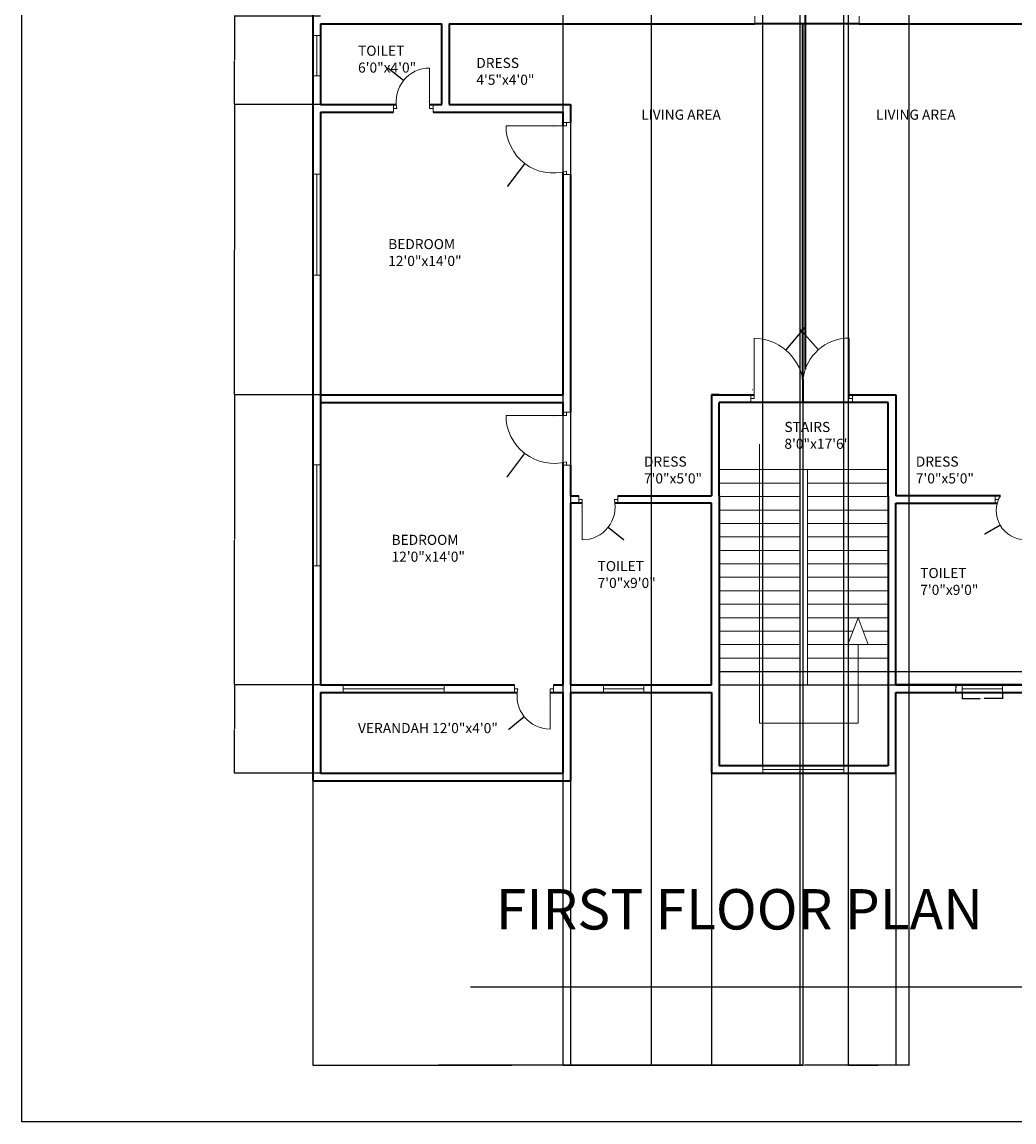
# Model space of a CAD drawing. Units: inches. Extents: x 1865 to 2795, y 1308 to 2437.
# Tile 1 of 3: x 1865 to 2455, y 1308 to 1962. Entities that reach past the tile are written whole.
import ezdxf

# ---------------------------------------------------------------- set-up
doc = ezdxf.new("R2010")
doc.units = ezdxf.units.IN
for name, color, linetype, lineweight in [('A-ANNO-DIMS', 2, 'Continuous', 18), ('A-ANNO-SYMB', 2, 'Continuous', 18), ('A-ANNO-TTLB', 7, 'Continuous', 25), ('A-AREA-IDEN', 7, 'Continuous', 18), ('A-DOOR', 3, 'Continuous', 18), ('A-FLOR-STRS', 7, 'Continuous', 18), ('A-GLAZ', 4, 'Continuous', 18), ('A-WALL', 7, 'Continuous', 35)]:
    doc.layers.add(name, color=color, linetype=linetype, lineweight=lineweight)
doc.styles.get("Standard").update_dxf_attribs({"font": 'arial.ttf'})
doc.dimstyles.get("Standard").update_dxf_attribs({"dimtxt": 0.18, "dimasz": 0.18, "dimexe": 0.18, "dimexo": 0.0625, "dimgap": 0.09, "dimtad": 0, "dimtih": 1, "dimtoh": 1, "dimdec": 4, "dimzin": 0, "dimdsep": 46, "dimtxsty": 'Standard', "dimcen": 0.09, "dimadec": 0, "dimazin": 0, "dimtfac": 1, "dimtdec": 4, "dimtofl": 0, "dimtmove": 0, "dimatfit": 3, "dimfxl": 1, "dimtolj": 1, "dimtzin": 0, "dimarcsym": 0})

# ---------------------------------------------------------------- blocks, each defined once
blk = doc.blocks.new('WIN-60IN')
for p, q in [((0, 4.5), (0, 0)), ((0, 0), (0, 2.25)), ((0, 2.25), (60, 2.25)), ((60, 2.25), (60, 4.5)), ((60, 4.5), (60, 0))]:
    blk.add_line(p, q)
blk = doc.blocks.new('WIN-60IN-ALT')
for p, q in [((4.5, 60), (0, 60)), ((0, 60), (2.25, 60)), ((2.25, 60), (2.25, 0)), ((2.25, 0), (0, 0)), ((0, 0), (4.5, 0))]:
    blk.add_line(p, q)
blk = doc.blocks.new('WIN-24IN')
for p, q in [((0, 24), (4.5, 24)), ((4.5, 24), (2.25, 24)), ((2.25, 24), (2.25, 0)), ((2.25, 0), (0, 0)), ((0, 0), (4.5, 0))]:
    blk.add_line(p, q)
blk = doc.blocks.new('*D6')
at = {"layer": 'A-ANNO-DIMS', "color": 0, "lineweight": -2, "transparency": 16777216}
for p, q in [((2424.19, 1563.59), (2424.19, 1559.88)), ((2448.19, 1563.59), (2448.19, 1559.88)), ((2424.37, 1560.06), (2435.07, 1560.06)), ((2448.01, 1560.06), (2437.31, 1560.06))]:
    blk.add_line(p, q, dxfattribs=at)
at = {"layer": 'A-ANNO-DIMS', "color": 0, "transparency": 16777216}
for points in [[(2424.37, 1560.09), (2424.37, 1560.03), (2424.19, 1560.06)], [(2448.01, 1560.09), (2448.01, 1560.03), (2448.19, 1560.06)]]:
    blk.add_solid(points, dxfattribs=at)
at = {"layer": 'Defpoints', "color": 0, "transparency": 16777216}
for p in [(2424.19, 1563.66), (2448.19, 1563.66), (2448.19, 1560.06)]:
    blk.add_point(p, dxfattribs=at)
at = {"layer": 'A-ANNO-DIMS', "color": 0, "transparency": 16777216, "insert": (2436.19, 1560.06), "char_height": 0.18, "attachment_point": 5}
blk.add_mtext('\\A1;WINDOW 24 TYP.', dxfattribs=at)
blk = doc.blocks.new('*D7')
at = {"layer": 'A-ANNO-DIMS', "color": 0, "lineweight": -2, "transparency": 16777216}
for p, q in [((2424.13, 1568.16), (2420.41, 1568.16)), ((2424.13, 1563.66), (2420.41, 1563.66)), ((2420.59, 1567.98), (2420.59, 1566.09)), ((2420.59, 1563.84), (2420.59, 1565.72))]:
    blk.add_line(p, q, dxfattribs=at)
at = {"layer": 'A-ANNO-DIMS', "color": 0, "transparency": 16777216}
for points in [[(2420.56, 1567.98), (2420.62, 1567.98), (2420.59, 1568.16)], [(2420.56, 1563.84), (2420.62, 1563.84), (2420.59, 1563.66)]]:
    blk.add_solid(points, dxfattribs=at)
at = {"layer": 'Defpoints', "color": 0, "transparency": 16777216}
for p in [(2420.59, 1563.66), (2424.19, 1568.16), (2424.19, 1563.66)]:
    blk.add_point(p, dxfattribs=at)
at = {"layer": 'A-ANNO-DIMS', "color": 0, "transparency": 16777216, "insert": (2420.59, 1565.91), "char_height": 0.18, "attachment_point": 5}
blk.add_mtext('\\A1;5 TYP.', dxfattribs=at)
blk = doc.blocks.new('*D12')
at = {"layer": 'A-ANNO-DIMS', "color": 0, "lineweight": -2, "transparency": 16777216}
for p, q in [((2038.34, 2310.59), (2038.34, 1341.86)), ((2186.84, 2306.09), (2186.84, 1341.86)), ((2038.52, 1342.04), (2112.2, 1342.04)), ((2186.66, 1342.04), (2112.97, 1342.04))]:
    blk.add_line(p, q, dxfattribs=at)
at = {"layer": 'A-ANNO-DIMS', "color": 0, "transparency": 16777216}
for points in [[(2038.52, 1342.07), (2038.52, 1342.01), (2038.34, 1342.04)], [(2186.66, 1342.07), (2186.66, 1342.01), (2186.84, 1342.04)]]:
    blk.add_solid(points, dxfattribs=at)
at = {"layer": 'Defpoints', "color": 0, "transparency": 16777216}
for p in [(2038.34, 2310.66), (2186.84, 2306.16), (2186.84, 1342.04)]:
    blk.add_point(p, dxfattribs=at)
at = {"layer": 'A-ANNO-DIMS', "color": 0, "transparency": 16777216, "insert": (2112.59, 1342.04), "char_height": 0.18, "attachment_point": 5}
blk.add_mtext('\\A1;148.5', dxfattribs=at)
blk = doc.blocks.new('*D13')
at = {"layer": 'A-ANNO-DIMS', "color": 0, "lineweight": -2, "transparency": 16777216}
for p, q in [((2186.84, 2306.09), (2186.84, 1341.86)), ((2239.34, 2306.09), (2239.34, 1341.86)), ((2187.02, 1342.04), (2212.76, 1342.04)), ((2239.16, 1342.04), (2213.41, 1342.04))]:
    blk.add_line(p, q, dxfattribs=at)
at = {"layer": 'A-ANNO-DIMS', "color": 0, "transparency": 16777216}
for points in [[(2187.02, 1342.07), (2187.02, 1342.01), (2186.84, 1342.04)], [(2239.16, 1342.07), (2239.16, 1342.01), (2239.34, 1342.04)]]:
    blk.add_solid(points, dxfattribs=at)
at = {"layer": 'Defpoints', "color": 0, "transparency": 16777216}
for p in [(2186.84, 2306.16), (2239.34, 2306.16), (2239.34, 1342.04)]:
    blk.add_point(p, dxfattribs=at)
at = {"layer": 'A-ANNO-DIMS', "color": 0, "transparency": 16777216, "insert": (2213.09, 1342.04), "char_height": 0.18, "attachment_point": 5}
blk.add_mtext('\\A1;52.5', dxfattribs=at)
blk = doc.blocks.new('*D14')
at = {"layer": 'A-ANNO-DIMS', "color": 0, "lineweight": -2, "transparency": 16777216}
for p, q in [((2239.34, 2306.09), (2239.34, 1341.86)), ((2327.84, 2306.09), (2327.84, 1341.86)), ((2239.52, 1342.04), (2283.26, 1342.04)), ((2327.66, 1342.04), (2283.91, 1342.04))]:
    blk.add_line(p, q, dxfattribs=at)
at = {"layer": 'A-ANNO-DIMS', "color": 0, "transparency": 16777216}
for points in [[(2239.52, 1342.07), (2239.52, 1342.01), (2239.34, 1342.04)], [(2327.66, 1342.07), (2327.66, 1342.01), (2327.84, 1342.04)]]:
    blk.add_solid(points, dxfattribs=at)
at = {"layer": 'Defpoints', "color": 0, "transparency": 16777216}
for p in [(2239.34, 2306.16), (2327.84, 2306.16), (2327.84, 1342.04)]:
    blk.add_point(p, dxfattribs=at)
at = {"layer": 'A-ANNO-DIMS', "color": 0, "transparency": 16777216, "insert": (2283.59, 1342.04), "char_height": 0.18, "attachment_point": 5}
blk.add_mtext('\\A1;88.5', dxfattribs=at)
blk = doc.blocks.new('*D18')
at = {"layer": 'A-ANNO-DIMS', "color": 0, "lineweight": -2, "transparency": 16777216}
for p, q in [((2356.56, 2306.09), (2356.56, 1341.86)), ((2392.56, 2306.09), (2392.56, 1341.86)), ((2356.74, 1342.04), (2374.34, 1342.04)), ((2392.38, 1342.04), (2374.78, 1342.04))]:
    blk.add_line(p, q, dxfattribs=at)
at = {"layer": 'A-ANNO-DIMS', "color": 0, "transparency": 16777216}
for points in [[(2356.74, 1342.07), (2356.74, 1342.01), (2356.56, 1342.04)], [(2392.38, 1342.07), (2392.38, 1342.01), (2392.56, 1342.04)]]:
    blk.add_solid(points, dxfattribs=at)
at = {"layer": 'Defpoints', "color": 0, "transparency": 16777216}
for p in [(2356.56, 2306.16), (2392.56, 2306.16), (2392.56, 1342.04)]:
    blk.add_point(p, dxfattribs=at)
at = {"layer": 'A-ANNO-DIMS', "color": 0, "transparency": 16777216, "insert": (2374.56, 1342.04), "char_height": 0.18, "attachment_point": 5}
blk.add_mtext('\\A1;36', dxfattribs=at)
blk = doc.blocks.new('*D19')
at = {"layer": 'A-ANNO-DIMS', "color": 0, "lineweight": -2, "transparency": 16777216}
for p, q in [((2305.85, 1520.22), (2305.85, 2357.44)), ((2306.03, 2357.26), (2329.63, 2357.26)), ((2353.67, 2357.26), (2330.08, 2357.26)), ((2353.85, 1520.22), (2353.85, 2357.44))]:
    blk.add_line(p, q, dxfattribs=at)
at = {"layer": 'A-ANNO-DIMS', "color": 0, "transparency": 16777216}
for points in [[(2306.03, 2357.29), (2306.03, 2357.23), (2305.85, 2357.26)], [(2353.67, 2357.29), (2353.67, 2357.23), (2353.85, 2357.26)]]:
    blk.add_solid(points, dxfattribs=at)
at = {"layer": 'Defpoints', "color": 0, "transparency": 16777216}
for p in [(2353.85, 2357.26), (2305.85, 1520.16), (2353.85, 1520.16)]:
    blk.add_point(p, dxfattribs=at)
at = {"layer": 'A-ANNO-DIMS', "color": 0, "transparency": 16777216, "insert": (2329.85, 2357.26), "char_height": 0.18, "attachment_point": 5}
blk.add_mtext('\\A1;48', dxfattribs=at)
blk = doc.blocks.new('*D20')
at = {"layer": 'A-ANNO-DIMS', "color": 0, "lineweight": -2, "transparency": 16777216}
for p, q in [((2042.78, 1568.16), (1991.56, 1568.16)), ((1991.74, 1567.98), (1991.74, 1542.09)), ((1991.74, 1515.84), (1991.74, 1541.72)), ((2042.78, 1515.66), (1991.56, 1515.66))]:
    blk.add_line(p, q, dxfattribs=at)
at = {"layer": 'A-ANNO-DIMS', "color": 0, "transparency": 16777216}
for points in [[(1991.71, 1567.98), (1991.77, 1567.98), (1991.74, 1568.16)], [(1991.71, 1515.84), (1991.77, 1515.84), (1991.74, 1515.66)]]:
    blk.add_solid(points, dxfattribs=at)
at = {"layer": 'Defpoints', "color": 0, "transparency": 16777216}
for p in [(1991.74, 1568.16), (2042.84, 1568.16), (2042.84, 1515.66)]:
    blk.add_point(p, dxfattribs=at)
at = {"layer": 'A-ANNO-DIMS', "color": 0, "transparency": 16777216, "insert": (1991.74, 1541.91), "char_height": 0.18, "attachment_point": 5}
blk.add_mtext('\\A1;52.5', dxfattribs=at)
blk = doc.blocks.new('*D21')
at = {"layer": 'A-ANNO-DIMS', "color": 0, "lineweight": -2, "transparency": 16777216}
for p, q in [((2042.78, 1740.66), (1991.56, 1740.66)), ((1991.74, 1740.48), (1991.74, 1654.59)), ((1991.74, 1568.34), (1991.74, 1654.22)), ((2042.78, 1568.16), (1991.56, 1568.16))]:
    blk.add_line(p, q, dxfattribs=at)
at = {"layer": 'A-ANNO-DIMS', "color": 0, "transparency": 16777216}
for points in [[(1991.71, 1740.48), (1991.77, 1740.48), (1991.74, 1740.66)], [(1991.71, 1568.34), (1991.77, 1568.34), (1991.74, 1568.16)]]:
    blk.add_solid(points, dxfattribs=at)
at = {"layer": 'Defpoints', "color": 0, "transparency": 16777216}
for p in [(1991.74, 1740.66), (2042.84, 1740.66), (2042.84, 1568.16)]:
    blk.add_point(p, dxfattribs=at)
at = {"layer": 'A-ANNO-DIMS', "color": 0, "transparency": 16777216, "insert": (1991.74, 1654.41), "char_height": 0.18, "attachment_point": 5}
blk.add_mtext('\\A1;172.5', dxfattribs=at)
blk = doc.blocks.new('*D22')
at = {"layer": 'A-ANNO-DIMS', "color": 0, "lineweight": -2, "transparency": 16777216}
for p, q in [((2042.78, 1913.16), (1991.56, 1913.16)), ((1991.74, 1912.98), (1991.74, 1827.09)), ((1991.74, 1740.84), (1991.74, 1826.72)), ((2042.78, 1740.66), (1991.56, 1740.66))]:
    blk.add_line(p, q, dxfattribs=at)
at = {"layer": 'A-ANNO-DIMS', "color": 0, "transparency": 16777216}
for points in [[(1991.71, 1912.98), (1991.77, 1912.98), (1991.74, 1913.16)], [(1991.71, 1740.84), (1991.77, 1740.84), (1991.74, 1740.66)]]:
    blk.add_solid(points, dxfattribs=at)
at = {"layer": 'Defpoints', "color": 0, "transparency": 16777216}
for p in [(1991.74, 1913.16), (2042.84, 1913.16), (2042.84, 1740.66)]:
    blk.add_point(p, dxfattribs=at)
at = {"layer": 'A-ANNO-DIMS', "color": 0, "transparency": 16777216, "insert": (1991.74, 1826.91), "char_height": 0.18, "attachment_point": 5}
blk.add_mtext('\\A1;172.5', dxfattribs=at)
blk = doc.blocks.new('*D23')
at = {"layer": 'A-ANNO-DIMS', "color": 0, "lineweight": -2, "transparency": 16777216}
for p, q in [((2042.78, 1965.66), (1991.56, 1965.66)), ((1991.74, 1965.48), (1991.74, 1939.59)), ((1991.74, 1913.34), (1991.74, 1939.22)), ((2042.78, 1913.16), (1991.56, 1913.16))]:
    blk.add_line(p, q, dxfattribs=at)
at = {"layer": 'A-ANNO-DIMS', "color": 0, "transparency": 16777216}
for points in [[(1991.71, 1965.48), (1991.77, 1965.48), (1991.74, 1965.66)], [(1991.71, 1913.34), (1991.77, 1913.34), (1991.74, 1913.16)]]:
    blk.add_solid(points, dxfattribs=at)
at = {"layer": 'Defpoints', "color": 0, "transparency": 16777216}
for p in [(1991.74, 1965.66), (2042.84, 1965.66), (2042.84, 1913.16)]:
    blk.add_point(p, dxfattribs=at)
at = {"layer": 'A-ANNO-DIMS', "color": 0, "transparency": 16777216, "insert": (1991.74, 1939.41), "char_height": 0.18, "attachment_point": 5}
blk.add_mtext('\\A1;52.5', dxfattribs=at)
blk = doc.blocks.new('*D25')
at = {"layer": 'A-ANNO-DIMS', "color": 0, "lineweight": -2, "transparency": 16777216}
for p, q in [((2038.34, 1511.09), (2038.34, 1341.86)), ((2275.34, 1515.59), (2275.34, 1341.86)), ((2038.52, 1342.04), (2156.55, 1342.04)), ((2275.16, 1342.04), (2157.13, 1342.04))]:
    blk.add_line(p, q, dxfattribs=at)
at = {"layer": 'A-ANNO-DIMS', "color": 0, "transparency": 16777216}
for points in [[(2038.52, 1342.07), (2038.52, 1342.01), (2038.34, 1342.04)], [(2275.16, 1342.07), (2275.16, 1342.01), (2275.34, 1342.04)]]:
    blk.add_solid(points, dxfattribs=at)
at = {"layer": 'Defpoints', "color": 0, "transparency": 16777216}
for p in [(2038.34, 1511.16), (2275.34, 1515.66), (2275.34, 1342.04)]:
    blk.add_point(p, dxfattribs=at)
at = {"layer": 'A-ANNO-DIMS', "color": 0, "transparency": 16777216, "insert": (2156.84, 1342.04), "char_height": 0.18, "attachment_point": 5}
blk.add_mtext('\\A1;237', dxfattribs=at)
blk = doc.blocks.new('*D26')
at = {"layer": 'A-ANNO-DIMS', "color": 0, "lineweight": -2, "transparency": 16777216}
for p, q in [((2275.34, 1515.59), (2275.34, 1341.86)), ((2384.84, 1515.59), (2384.84, 1341.86)), ((2275.52, 1342.04), (2329.7, 1342.04)), ((2384.66, 1342.04), (2330.47, 1342.04))]:
    blk.add_line(p, q, dxfattribs=at)
at = {"layer": 'A-ANNO-DIMS', "color": 0, "transparency": 16777216}
for points in [[(2275.52, 1342.07), (2275.52, 1342.01), (2275.34, 1342.04)], [(2384.66, 1342.07), (2384.66, 1342.01), (2384.84, 1342.04)]]:
    blk.add_solid(points, dxfattribs=at)
at = {"layer": 'Defpoints', "color": 0, "transparency": 16777216}
for p in [(2275.34, 1515.66), (2384.84, 1515.66), (2384.84, 1342.04)]:
    blk.add_point(p, dxfattribs=at)
at = {"layer": 'A-ANNO-DIMS', "color": 0, "transparency": 16777216, "insert": (2330.09, 1342.04), "char_height": 0.18, "attachment_point": 5}
blk.add_mtext('\\A1;109.5', dxfattribs=at)
blk = doc.blocks.new('*D27')
at = {"layer": 'A-ANNO-DIMS', "color": 0, "lineweight": -2, "transparency": 16777216}
for p, q in [((2329.63, 1961.09), (2329.63, 1341.86)), ((2191.34, 1913.09), (2191.34, 1341.86)), ((2191.52, 1342.04), (2260.1, 1342.04)), ((2329.45, 1342.04), (2260.87, 1342.04))]:
    blk.add_line(p, q, dxfattribs=at)
at = {"layer": 'A-ANNO-DIMS', "color": 0, "transparency": 16777216}
for points in [[(2191.52, 1342.07), (2191.52, 1342.01), (2191.34, 1342.04)], [(2329.45, 1342.07), (2329.45, 1342.01), (2329.63, 1342.04)]]:
    blk.add_solid(points, dxfattribs=at)
at = {"layer": 'Defpoints', "color": 0, "transparency": 16777216}
for p in [(2329.63, 1961.16), (2191.34, 1913.16), (2329.63, 1342.04)]:
    blk.add_point(p, dxfattribs=at)
at = {"layer": 'A-ANNO-DIMS', "color": 0, "transparency": 16777216, "insert": (2260.48, 1342.04), "char_height": 0.18, "attachment_point": 5}
blk.add_mtext('\\A1;138.3', dxfattribs=at)
blk = doc.blocks.new('*D28')
at = {"layer": 'A-ANNO-DIMS', "color": 0, "lineweight": -2, "transparency": 16777216}
for p, q in [((2279.9, 1576.16), (2668.62, 1576.16)), ((2668.44, 1575.98), (2668.44, 1572.34)), ((2668.44, 1568.34), (2668.44, 1571.97)), ((2279.9, 1568.16), (2668.62, 1568.16))]:
    blk.add_line(p, q, dxfattribs=at)
at = {"layer": 'A-ANNO-DIMS', "color": 0, "transparency": 16777216}
for points in [[(2668.41, 1575.98), (2668.47, 1575.98), (2668.44, 1576.16)], [(2668.41, 1568.34), (2668.47, 1568.34), (2668.44, 1568.16)]]:
    blk.add_solid(points, dxfattribs=at)
at = {"layer": 'Defpoints', "color": 0, "transparency": 16777216}
for p in [(2279.84, 1576.16), (2668.44, 1576.16), (2279.84, 1568.16)]:
    blk.add_point(p, dxfattribs=at)
at = {"layer": 'A-ANNO-DIMS', "color": 0, "transparency": 16777216, "insert": (2668.44, 1572.16), "char_height": 0.18, "attachment_point": 5}
blk.add_mtext('\\A1;8', dxfattribs=at)
blk = doc.blocks.new('*D30')
at = {"layer": 'A-ANNO-DIMS', "color": 0, "lineweight": -2, "transparency": 16777216}
for p, q in [((2331.21, 1781.26), (2319.48, 1767.35)), ((2331.39, 1781.26), (2331.21, 1781.26)), ((2299.55, 1743.81), (2299.73, 1743.81)), ((2299.64, 1743.72), (2299.64, 1743.9))]:
    blk.add_line(p, q, dxfattribs=at)
at = {"layer": 'A-ANNO-DIMS', "color": 0, "transparency": 16777216}
blk.add_solid([(2319.46, 1767.37), (2319.51, 1767.34), (2319.37, 1767.22)], dxfattribs=at)
at = {"layer": 'Defpoints', "color": 0, "transparency": 16777216}
for p in [(2319.37, 1767.22), (2299.64, 1743.81)]:
    blk.add_point(p, dxfattribs=at)
at = {"layer": 'A-ANNO-DIMS', "color": 0, "transparency": 16777216, "insert": (2331.85, 1781.26), "char_height": 0.18, "attachment_point": 5}
blk.add_mtext('\\A1;R30.61', dxfattribs=at)
blk = doc.blocks.new('*D34')
at = {"layer": 'A-ANNO-DIMS', "color": 0, "lineweight": -2, "transparency": 16777216}
for p, q in [((2181.53, 1728.42), (2181.71, 1728.42)), ((2181.62, 1728.33), (2181.62, 1728.51)), ((2153.89, 1692.16), (2164.18, 1705.61)), ((2153.71, 1692.16), (2153.89, 1692.16))]:
    blk.add_line(p, q, dxfattribs=at)
at = {"layer": 'A-ANNO-DIMS', "color": 0, "transparency": 16777216}
blk.add_solid([(2164.15, 1705.63), (2164.2, 1705.59), (2164.29, 1705.76)], dxfattribs=at)
at = {"layer": 'Defpoints', "color": 0, "transparency": 16777216}
for p in [(2181.62, 1728.42), (2164.29, 1705.76)]:
    blk.add_point(p, dxfattribs=at)
at = {"layer": 'A-ANNO-DIMS', "color": 0, "transparency": 16777216, "insert": (2153.23, 1692.16), "char_height": 0.18, "attachment_point": 5}
blk.add_mtext('\\A1;R28.53', dxfattribs=at)
blk = doc.blocks.new('*D36')
at = {"layer": 'A-ANNO-DIMS', "color": 0, "lineweight": -2, "transparency": 16777216}
for p, q in [((2181.07, 1900.57), (2181.25, 1900.57)), ((2181.16, 1900.48), (2181.16, 1900.66)), ((2154.25, 1864.6), (2164.24, 1877.95)), ((2154.07, 1864.6), (2154.25, 1864.6))]:
    blk.add_line(p, q, dxfattribs=at)
at = {"layer": 'A-ANNO-DIMS', "color": 0, "transparency": 16777216}
blk.add_solid([(2164.21, 1877.96), (2164.26, 1877.93), (2164.34, 1878.09)], dxfattribs=at)
at = {"layer": 'Defpoints', "color": 0, "transparency": 16777216}
for p in [(2181.16, 1900.57), (2164.34, 1878.09)]:
    blk.add_point(p, dxfattribs=at)
at = {"layer": 'A-ANNO-DIMS', "color": 0, "transparency": 16777216, "insert": (2153.52, 1864.6), "char_height": 0.18, "attachment_point": 5}
blk.add_mtext('\\A1;R28.075', dxfattribs=at)
blk = doc.blocks.new('*D38')
at = {"layer": 'A-ANNO-DIMS', "color": 0, "lineweight": -2, "transparency": 16777216}
for p, q in [((2327.53, 1779.86), (2327.71, 1779.86)), ((2327.71, 1779.86), (2338.64, 1767.55)), ((2357.08, 1746.67), (2357.26, 1746.67)), ((2357.17, 1746.58), (2357.17, 1746.76))]:
    blk.add_line(p, q, dxfattribs=at)
at = {"layer": 'A-ANNO-DIMS', "color": 0, "transparency": 16777216}
blk.add_solid([(2338.66, 1767.57), (2338.61, 1767.53), (2338.76, 1767.42)], dxfattribs=at)
at = {"layer": 'Defpoints', "color": 0, "transparency": 16777216}
for p in [(2338.76, 1767.42), (2357.17, 1746.67)]:
    blk.add_point(p, dxfattribs=at)
at = {"layer": 'A-ANNO-DIMS', "color": 0, "transparency": 16777216, "insert": (2327.05, 1779.86), "char_height": 0.18, "attachment_point": 5}
blk.add_mtext('\\A1;R27.74', dxfattribs=at)
blk = doc.blocks.new('*D44')
at = {"layer": 'A-ANNO-DIMS', "color": 0, "lineweight": -2, "transparency": 16777216}
for p, q in [((2082.75, 1935.12), (2082.93, 1935.12)), ((2082.93, 1935.12), (2092.08, 1927.67)), ((2107.6, 1914.94), (2107.78, 1914.94)), ((2107.69, 1914.85), (2107.69, 1915.03))]:
    blk.add_line(p, q, dxfattribs=at)
at = {"layer": 'A-ANNO-DIMS', "color": 0, "transparency": 16777216}
blk.add_solid([(2092.09, 1927.69), (2092.06, 1927.64), (2092.22, 1927.55)], dxfattribs=at)
at = {"layer": 'Defpoints', "color": 0, "transparency": 16777216}
for p in [(2092.22, 1927.55), (2107.69, 1914.94)]:
    blk.add_point(p, dxfattribs=at)
at = {"layer": 'A-ANNO-DIMS', "color": 0, "transparency": 16777216, "insert": (2082.2, 1935.12), "char_height": 0.18, "attachment_point": 5}
blk.add_mtext('\\A1;R19.965', dxfattribs=at)
blk = doc.blocks.new('*D45')
at = {"layer": 'A-ANNO-DIMS', "color": 0, "lineweight": -2, "transparency": 16777216}
for p, q in [((2198.34, 1673.97), (2198.34, 1674.15)), ((2198.25, 1674.06), (2198.43, 1674.06)), ((2222.91, 1654.44), (2213.84, 1661.68)), ((2223.09, 1654.44), (2222.91, 1654.44))]:
    blk.add_line(p, q, dxfattribs=at)
at = {"layer": 'A-ANNO-DIMS', "color": 0, "transparency": 16777216}
blk.add_solid([(2213.86, 1661.71), (2213.82, 1661.66), (2213.7, 1661.8)], dxfattribs=at)
at = {"layer": 'Defpoints', "color": 0, "transparency": 16777216}
for p in [(2198.34, 1674.06), (2213.7, 1661.8)]:
    blk.add_point(p, dxfattribs=at)
at = {"layer": 'A-ANNO-DIMS', "color": 0, "transparency": 16777216, "insert": (2223.57, 1654.44), "char_height": 0.18, "attachment_point": 5}
blk.add_mtext('\\A1;R19.65', dxfattribs=at)
blk = doc.blocks.new('*D46')
at = {"layer": 'A-ANNO-DIMS', "color": 0, "lineweight": -2, "transparency": 16777216}
for p, q in [((2179.17, 1561.52), (2179.35, 1561.52)), ((2179.26, 1561.43), (2179.26, 1561.61)), ((2154.72, 1541.97), (2163.78, 1549.19)), ((2154.54, 1541.97), (2154.72, 1541.97))]:
    blk.add_line(p, q, dxfattribs=at)
at = {"layer": 'A-ANNO-DIMS', "color": 0, "transparency": 16777216}
blk.add_solid([(2163.76, 1549.21), (2163.8, 1549.16), (2163.92, 1549.3)], dxfattribs=at)
at = {"layer": 'Defpoints', "color": 0, "transparency": 16777216}
for p in [(2179.26, 1561.52), (2163.92, 1549.3)]:
    blk.add_point(p, dxfattribs=at)
at = {"layer": 'A-ANNO-DIMS', "color": 0, "transparency": 16777216, "insert": (2153.99, 1541.97), "char_height": 0.18, "attachment_point": 5}
blk.add_mtext('\\A1;R19.615', dxfattribs=at)
blk = doc.blocks.new('*D49')
at = {"layer": 'A-ANNO-DIMS', "color": 0, "lineweight": -2, "transparency": 16777216}
for p, q in [((2461.87, 1671.78), (2462.05, 1671.78)), ((2461.96, 1671.69), (2461.96, 1671.87)), ((2437.81, 1658.01), (2446.71, 1663.08)), ((2437.63, 1658.01), (2437.81, 1658.01))]:
    blk.add_line(p, q, dxfattribs=at)
at = {"layer": 'A-ANNO-DIMS', "color": 0, "transparency": 16777216}
blk.add_solid([(2446.7, 1663.11), (2446.73, 1663.06), (2446.87, 1663.17)], dxfattribs=at)
at = {"layer": 'Defpoints', "color": 0, "transparency": 16777216}
for p in [(2461.96, 1671.78), (2446.87, 1663.17)]:
    blk.add_point(p, dxfattribs=at)
at = {"layer": 'A-ANNO-DIMS', "color": 0, "transparency": 16777216, "insert": (2437.09, 1658.01), "char_height": 0.18, "attachment_point": 5}
blk.add_mtext('\\A1;R17.372', dxfattribs=at)

msp = doc.modelspace()

# ---------------------------------------------------------------- linework, layer by layer
at = {"layer": 'A-ANNO-SYMB'}
for p, q in [((2303.8379, 1711.3839), (2303.8379, 1545.3723)), ((2362.5426, 1608.1564), (2356.3379, 1592.1564)), ((2368.4808, 1592.1564), (2362.5426, 1608.1564)), ((2356.3379, 1592.1564), (2368.4808, 1592.1564)), ((2362.5426, 1545.3723), (2362.5426, 1592.1564)), ((2303.8379, 1545.3723), (2362.5426, 1545.3723))]:
    msp.add_line(p, q, dxfattribs=at)
at = {"layer": 'A-ANNO-TTLB'}
msp.add_line((2132.0289, 1388.6384), (2475.3371, 1388.6384), dxfattribs=at)
msp.add_lwpolyline([(1865.3404, 2436.9121), (2795.2369, 2436.9121), (2795.2369, 1308.3367), (1865.3404, 1308.3367)], close=True, dxfattribs=at)
at = {"layer": 'A-DOOR'}
for p, q in [((2301.0168, 1965.6564), (2301.0168, 1961.1564)), ((2301.0168, 1961.1564), (2301.0168, 1963.4064)), ((2363.0176, 1965.6564), (2363.0176, 1961.1564)), ((2363.0176, 1961.1564), (2363.0176, 1963.4064)), ((2107.6934, 1910.9064), (2107.6934, 1934.9064)), ((2086.1404, 1913.1564), (2086.1404, 1908.6564)), ((2086.1404, 1908.6564), (2086.1404, 1910.9064)), ((2086.1404, 1910.9064), (2088.1404, 1910.9064)), ((2109.6934, 1910.9064), (2107.6934, 1910.9064)), ((2109.6934, 1913.1564), (2109.6934, 1908.6564)), ((2109.6934, 1908.6564), (2109.6934, 1910.9064)), ((2189.0879, 1900.57), (2153.0879, 1900.57)), ((2186.8379, 1902.57), (2191.3379, 1902.57)), ((2191.3379, 1902.57), (2189.0879, 1902.57)), ((2189.0879, 1902.57), (2189.0879, 1900.57)), ((2186.8379, 1871.6368), (2191.3379, 1871.6368)), ((2189.0879, 1871.6368), (2189.0879, 1873.6368)), ((2191.3379, 1871.6368), (2189.0879, 1871.6368)), ((2300.6319, 1738.4064), (2300.6319, 1774.4064)), ((2357.1665, 1738.4064), (2357.1665, 1774.4064)), ((2298.6319, 1740.6564), (2298.6319, 1736.1564)), ((2359.1665, 1740.6564), (2359.1665, 1736.1564)), ((2298.6319, 1736.1564), (2298.6319, 1738.4064)), ((2298.6319, 1738.4064), (2300.6319, 1738.4064)), ((2359.1665, 1738.4064), (2357.1665, 1738.4064)), ((2359.1665, 1736.1564), (2359.1665, 1738.4064)), ((2189.0879, 1728.4167), (2153.0879, 1728.4167)), ((2186.8379, 1730.4167), (2191.3379, 1730.4167)), ((2191.3379, 1730.4167), (2189.0879, 1730.4167)), ((2189.0879, 1730.4167), (2189.0879, 1728.4167)), ((2189.0879, 1698.8854), (2189.0879, 1700.8854)), ((2186.8379, 1698.8854), (2191.3379, 1698.8854)), ((2191.3379, 1698.8854), (2189.0879, 1698.8854)), ((2196.3405, 1680.6564), (2196.3405, 1676.1564)), ((2219.5026, 1676.1564), (2219.5026, 1680.6564)), ((2219.5026, 1680.6564), (2219.5026, 1678.4064)), ((2443.9024, 1676.1564), (2443.9024, 1680.6564)), ((2443.9024, 1680.6564), (2443.9024, 1678.4064)), ((2196.3405, 1676.1564), (2196.3405, 1678.4064)), ((2196.3405, 1678.4064), (2198.3405, 1678.4064)), ((2198.3405, 1678.4064), (2198.3405, 1654.4064)), ((2219.5026, 1678.4064), (2217.5026, 1678.4064)), ((2443.9024, 1678.4064), (2445.9024, 1678.4064)), ((2158.1451, 1568.1564), (2158.1451, 1563.6564)), ((2158.1451, 1563.6564), (2158.1451, 1565.9064)), ((2158.1451, 1565.9064), (2160.1451, 1565.9064)), ((2181.2633, 1565.9064), (2179.2633, 1565.9064)), ((2179.2633, 1565.9064), (2179.2633, 1541.9064)), ((2181.2633, 1568.1564), (2181.2633, 1563.6564)), ((2181.2633, 1563.6564), (2181.2633, 1565.9064))]:
    msp.add_line(p, q, dxfattribs=at)
for centre, radius, start, end in [((2303.4402, 1971.6481), 27.7616, 331.5011644, 331.5011645), ((2107.6934, 1914.9415), 19.965, 90, 191.6600786), ((2181.1628, 1900.57), 28.0749, 180, 286.3964485), ((2299.6392, 1743.8109), 30.6116, 11.6021049, 88.1416575), ((2357.1665, 1746.6684), 27.738, 90, 173.169599), ((2181.6152, 1728.4167), 28.5274, 180, 285.1854956), ((2461.9604, 1671.7785), 17.3721, 149.2662645, 270.1168983), ((2198.3405, 1674.0562), 19.6497, 270, 12.790729), ((2179.2633, 1561.5211), 19.6147, 167.0809417, 270)]:
    msp.add_arc(centre, radius, start, end, dxfattribs=at)
at = {"layer": 'A-FLOR-STRS'}
for p, q in [((2279.8379, 1696.1564), (2327.8379, 1696.1564)), ((2327.8379, 1696.1564), (2327.8379, 1568.1564)), ((2327.8379, 1696.1564), (2332.3379, 1696.1564)), ((2332.3379, 1696.1564), (2380.3379, 1696.1564)), ((2332.3379, 1696.1564), (2332.3379, 1568.1564)), ((2279.8379, 1688.1564), (2327.8379, 1688.1564)), ((2332.3379, 1688.1564), (2380.3379, 1688.1564)), ((2279.8379, 1680.1564), (2327.8379, 1680.1564)), ((2332.3379, 1680.1564), (2380.3379, 1680.1564)), ((2279.8379, 1672.1564), (2327.8379, 1672.1564)), ((2332.3379, 1672.1564), (2380.3379, 1672.1564)), ((2279.8379, 1664.1564), (2327.8379, 1664.1564)), ((2332.3379, 1664.1564), (2380.3379, 1664.1564)), ((2279.8379, 1656.1564), (2327.8379, 1656.1564)), ((2332.3379, 1656.1564), (2380.3379, 1656.1564)), ((2279.8379, 1648.1564), (2327.8379, 1648.1564)), ((2332.3379, 1648.1564), (2380.3379, 1648.1564)), ((2279.8379, 1640.1564), (2327.8379, 1640.1564)), ((2332.3379, 1640.1564), (2380.3379, 1640.1564)), ((2279.8379, 1632.1564), (2327.8379, 1632.1564)), ((2332.3379, 1632.1564), (2380.3379, 1632.1564)), ((2279.8379, 1624.1564), (2327.8379, 1624.1564)), ((2332.3379, 1624.1564), (2380.3379, 1624.1564)), ((2279.8379, 1616.1564), (2327.8379, 1616.1564)), ((2332.3379, 1616.1564), (2380.3379, 1616.1564)), ((2279.8379, 1608.1564), (2327.8379, 1608.1564)), ((2332.3379, 1608.1564), (2380.3379, 1608.1564)), ((2279.8379, 1600.1564), (2327.8379, 1600.1564)), ((2332.3379, 1600.1564), (2359.4402, 1600.1564)), ((2365.5117, 1600.1564), (2380.3379, 1600.1564)), ((2279.8379, 1592.1564), (2327.8379, 1592.1564)), ((2332.3379, 1592.1564), (2380.3379, 1592.1564)), ((2279.8379, 1584.1564), (2327.8379, 1584.1564)), ((2332.3379, 1584.1564), (2380.3379, 1584.1564)), ((2279.8379, 1576.1564), (2327.8379, 1576.1564)), ((2332.3379, 1576.1564), (2380.3379, 1576.1564)), ((2279.8379, 1568.1564), (2327.8379, 1568.1564)), ((2332.3379, 1568.1564), (2380.3379, 1568.1564))]:
    msp.add_line(p, q, dxfattribs=at)
at = {"layer": 'A-GLAZ'}
for p, q in [((2305.8539, 1520.1564), (2305.8539, 1515.6564)), ((2305.8539, 1515.6564), (2305.8539, 1517.9064)), ((2305.8539, 1517.9064), (2353.8539, 1517.9064)), ((2353.8539, 1517.9064), (2353.8539, 1520.1564)), ((2353.8539, 1520.1564), (2353.8539, 1515.6564))]:
    msp.add_line(p, q, dxfattribs=at)
at = {"layer": 'A-WALL'}
for p, q in [((2038.3379, 2310.6564), (2038.3379, 1511.1564)), ((2331.0091, 1974.9133), (2331.0091, 1961.1564)), ((2042.8379, 1961.1564), (2114.8379, 1961.1564)), ((2042.8379, 1961.1564), (2042.8379, 1913.1564)), ((2114.8379, 1913.1564), (2114.8379, 1961.1564)), ((2119.3379, 1961.1564), (2119.3379, 1913.1564)), ((2119.3379, 1961.1564), (2191.3379, 1961.1564)), ((2191.3379, 1961.1564), (2301.0168, 1961.1564)), ((2363.0176, 1961.1564), (2301.0168, 1961.1564)), ((2329.6254, 1749.9673), (2329.6254, 1961.1564)), ((2331.0091, 1961.1564), (2331.0197, 1755.9281)), ((2363.0176, 1961.1564), (2473.3379, 1961.1564)), ((2042.8379, 1913.1564), (2087.8084, 1913.1564)), ((2107.6934, 1913.1564), (2114.8379, 1913.1564)), ((2119.3379, 1913.1564), (2191.3379, 1913.1564)), ((2191.3379, 1913.1564), (2191.3379, 1902.57)), ((2042.8379, 1908.6564), (2086.1404, 1908.6564)), ((2042.8379, 1908.6564), (2086.1404, 1908.6564)), ((2042.8379, 1908.6564), (2042.8379, 1568.1564)), ((2109.6934, 1908.6564), (2114.8379, 1908.6564)), ((2109.6934, 1908.6564), (2186.8379, 1908.6564)), ((2186.8379, 1908.6564), (2186.8379, 1900.57)), ((2186.8379, 1873.0746), (2186.8379, 1740.6564)), ((2191.3379, 1871.6368), (2191.3379, 1730.4167)), ((2329.6254, 1749.9673), (2329.6254, 1736.1564)), ((2042.8379, 1740.6564), (2186.8379, 1740.6564)), ((2275.3379, 1740.6564), (2300.6319, 1740.6564)), ((2279.8379, 1740.6564), (2275.3379, 1740.6564)), ((2275.3379, 1740.6564), (2275.3379, 1680.6564)), ((2357.1665, 1740.6564), (2384.8379, 1740.6564)), ((2380.3379, 1740.6564), (2384.8379, 1740.6564)), ((2384.8379, 1740.6564), (2384.8379, 1680.6564)), ((2042.8379, 1736.1564), (2186.8379, 1736.1564)), ((2186.8379, 1736.1564), (2186.8379, 1728.4167)), ((2279.8379, 1680.6564), (2279.8379, 1736.1564)), ((2380.3379, 1736.1564), (2279.8379, 1736.1564)), ((2380.3379, 1680.6564), (2380.3379, 1736.1564)), ((2186.8379, 1700.3715), (2186.8379, 1568.1564)), ((2191.3379, 1698.8854), (2191.3379, 1680.6564)), ((2191.3379, 1680.6564), (2196.3405, 1680.6564)), ((2219.5026, 1680.6564), (2275.3379, 1680.6564)), ((2279.8379, 1680.6564), (2279.8379, 1568.1564)), ((2380.3379, 1680.6564), (2380.3379, 1568.1564)), ((2447.0282, 1680.6564), (2384.8379, 1680.6564)), ((2198.3405, 1676.1564), (2191.3379, 1676.1564)), ((2191.3379, 1676.1564), (2191.3379, 1568.1564)), ((2275.3379, 1676.1564), (2217.8776, 1676.1564)), ((2275.3379, 1568.1564), (2275.3379, 1676.1564)), ((2384.8379, 1568.1564), (2384.8379, 1676.1564)), ((2384.8379, 1676.1564), (2445.1491, 1676.1564)), ((2042.8379, 1568.1564), (2158.1451, 1568.1564)), ((2042.8379, 1563.6564), (2159.7652, 1563.6564)), ((2042.8379, 1563.6564), (2042.8379, 1515.6564)), ((2179.2633, 1563.6564), (2186.8379, 1563.6564)), ((2181.2633, 1568.1564), (2186.8379, 1568.1564)), ((2186.8379, 1563.6564), (2186.8379, 1515.6564)), ((2191.3379, 1568.1564), (2275.3379, 1568.1564)), ((2191.3379, 1568.1564), (2275.3379, 1568.1564)), ((2191.3379, 1563.6564), (2275.3379, 1563.6564)), ((2191.3379, 1563.6564), (2191.3379, 1511.1564)), ((2275.3379, 1563.6564), (2275.3379, 1515.6564)), ((2279.8379, 1568.1564), (2279.8379, 1520.1564)), ((2380.3379, 1568.1564), (2380.3379, 1520.1564)), ((2468.8379, 1568.1564), (2384.8379, 1568.1564)), ((2384.8379, 1568.1564), (2468.8379, 1568.1564)), ((2384.8379, 1515.6564), (2384.8379, 1563.6564)), ((2384.8379, 1563.6564), (2468.8379, 1563.6564)), ((2380.3379, 1520.1564), (2279.8379, 1520.1564)), ((2038.3379, 1511.1564), (2191.3379, 1511.1564)), ((2042.8379, 1515.6564), (2186.8379, 1515.6564)), ((2275.3379, 1515.6564), (2384.8379, 1515.6564))]:
    msp.add_line(p, q, dxfattribs=at)

# ---------------------------------------------------------------- block references
at = {"layer": 'A-GLAZ'}
for name, p in [('WIN-24IN', (2038.338, 1930.231)), ('WIN-60IN', (2056.2677, 1563.656))]:
    msp.add_blockref(name, p, dxfattribs=at)
at = {"layer": 'A-GLAZ', "extrusion": (0, 0, -1), "zscale": -1, "rotation": 270}
for name, p in [('WIN-60IN', (-2042.8383, 1871.8319)), ('WIN-24IN', (-2234.9534, 1568.1563))]:
    msp.add_blockref(name, p, dxfattribs=at)
at = {"layer": 'A-GLAZ', "extrusion": (0, 0, -1), "zscale": -1}
msp.add_blockref('WIN-60IN-ALT', (-2042.8377, 1638.9242), dxfattribs=at)
at = {"layer": 'A-GLAZ', "rotation": 270}
msp.add_blockref('WIN-24IN', (2424.1918, 1568.1563), dxfattribs=at)

# ---------------------------------------------------------------- texts
at = {"layer": 'A-ANNO-TTLB', "insert": (2147.0758, 1446.7791), "char_height": 24, "attachment_point": 1}
msp.add_mtext_dynamic_manual_height_columns('FIRST FLOOR PLAN', width=659.819803, gutter_width=12.5, heights=[0], dxfattribs=at)
at = {"layer": 'A-AREA-IDEN', "char_height": 6, "attachment_point": 1}
for s, width, insert in [('TOILET\\P6\'0"x4\'0"', 137.196169, (2065.1165, 1948.1847)), ('DRESS\\P4\'5"x4\'0"', 79.05405, (2135.4293, 1940.9443)), ('LIVING AREA', 149.040239, (2233.4769, 1910.1863)), ('LIVING AREA', 149.040239, (2373.0739, 1910.1863)), ('BEDROOM\\P12\'0"x14\'0"', 238.427555, (2083.0269, 1833.2426)), ('STAIRS \\P8\'0"x17\'6"', 112.257651, (2318.5984, 1724.5384)), ('DRESS\\P7\'0"x5\'0"', 97.973311, (2235.0857, 1703.9492)), ('DRESS\\P7\'0"x5\'0"', 97.973311, (2396.7292, 1703.9492)), ('BEDROOM\\P12\'0"x14\'0"', 271.171269, (2085.0253, 1657.4139)), ('TOILET\\P7\'0"x9\'0"', 185.000953, (2207.5379, 1641.8181)), ('TOILET\\P7\'0"x9\'0"', 120.921234, (2399.3393, 1637.7042)), ('VERANDAH 12\'0"x4\'0"', 199.483807, (2065.1116, 1545.5133))]:
    msp.add_mtext_dynamic_manual_height_columns(s, width=width, gutter_width=12.5, heights=[0], dxfattribs=dict(at, insert=insert))

# ---------------------------------------------------------------- dimensions: what is measured, and where the dimension line sits
at = {"layer": 'A-ANNO-DIMS'}
for base, p1, p2, override, picture, middle in [((2353.8539, 2357.2564), (2305.8539, 1520.1564), (2353.8539, 1520.1564), {"dimdec": 0, "dimlfac": 1, "dimrnd": 0, "dimzin": 0, "dimdsep": 46, "dimlunit": 2}, '*D19', (2329.8539, 2357.2564)), ((2186.8379, 1342.0384), (2038.3379, 2310.6564), (2186.8379, 2306.1564), {"dimdec": 1, "dimlfac": 1, "dimrnd": 0, "dimzin": 0, "dimdsep": 46, "dimlunit": 2}, '*D12', (2112.5879, 1342.0384)), ((2239.3379, 1342.0384), (2186.8379, 2306.1564), (2239.3379, 2306.1564), {"dimdec": 1, "dimlfac": 1, "dimrnd": 0, "dimzin": 0, "dimdsep": 46, "dimlunit": 2}, '*D13', (2213.0879, 1342.0384)), ((2327.8379, 1342.0384), (2239.3379, 2306.1564), (2327.8379, 2306.1564), {"dimdec": 1, "dimlfac": 1, "dimrnd": 0, "dimzin": 0, "dimdsep": 46, "dimlunit": 2}, '*D14', (2283.5879, 1342.0384)), ((2392.5618, 1342.0384), (2356.5618, 2306.1564), (2392.5618, 2306.1564), {"dimdec": 0, "dimlfac": 1, "dimrnd": 0, "dimzin": 0, "dimdsep": 46, "dimlunit": 2}, '*D18', (2374.5618, 1342.0384)), ((2329.6254, 1342.0384), (2191.3379, 1913.1564), (2329.6254, 1961.1564), {"dimdec": 1, "dimlfac": 1, "dimrnd": 0, "dimzin": 0, "dimdsep": 46, "dimlunit": 2}, '*D27', (2260.4816, 1342.0384)), ((2275.3379, 1342.0384), (2038.3379, 1511.1564), (2275.3379, 1515.6564), {"dimdec": 0, "dimlfac": 1, "dimrnd": 0, "dimzin": 0, "dimdsep": 46, "dimlunit": 2}, '*D25', (2156.8379, 1342.0384)), ((2384.8379, 1342.0384), (2275.3379, 1515.6564), (2384.8379, 1515.6564), {"dimdec": 1, "dimlfac": 1, "dimrnd": 0, "dimzin": 0, "dimdsep": 46, "dimlunit": 2}, '*D26', (2330.0879, 1342.0384))]:
    dim = msp.add_linear_dim(base=base, p1=p1, p2=p2, dimstyle='Standard', override=override, dxfattribs=at)
    dim.commit()
    dim.dimension.update_dxf_attribs({"geometry": picture, "text_midpoint": middle})
for base, p1, p2, override, picture, middle in [((1991.7379, 1965.6564), (2042.8379, 1913.1564), (2042.8379, 1965.6564), {"dimdec": 1, "dimlfac": 1, "dimrnd": 0, "dimzin": 0, "dimdsep": 46, "dimlunit": 2}, '*D23', (1991.7379, 1939.4064)), ((1991.7379, 1913.1564), (2042.8379, 1740.6564), (2042.8379, 1913.1564), {"dimdec": 1, "dimlfac": 1, "dimrnd": 0, "dimzin": 0, "dimdsep": 46, "dimlunit": 2}, '*D22', (1991.7379, 1826.9064)), ((1991.7379, 1740.6564), (2042.8379, 1568.1564), (2042.8379, 1740.6564), {"dimdec": 1, "dimlfac": 1, "dimrnd": 0, "dimzin": 0, "dimdsep": 46, "dimlunit": 2}, '*D21', (1991.7379, 1654.4064)), ((2668.4379, 1576.1564), (2279.8379, 1568.1564), (2279.8379, 1576.1564), {"dimdec": 0, "dimlfac": 1, "dimrnd": 0, "dimzin": 0, "dimdsep": 46, "dimlunit": 2}, '*D28', (2668.4379, 1572.1564)), ((1991.7379, 1568.1564), (2042.8379, 1515.6564), (2042.8379, 1568.1564), {"dimdec": 1, "dimlfac": 1, "dimrnd": 0, "dimzin": 0, "dimdsep": 46, "dimlunit": 2}, '*D20', (1991.7379, 1541.9064))]:
    dim = msp.add_linear_dim(base=base, p1=p1, p2=p2, angle=90, dimstyle='Standard', override=override, dxfattribs=at)
    dim.commit()
    dim.dimension.update_dxf_attribs({"geometry": picture, "text_midpoint": middle})
for center, mpoint, override, picture, middle in [((2107.6934, 1914.9415), (2092.2151, 1927.5519), {"dimdec": 3, "dimlfac": 1, "dimrnd": 0, "dimzin": 0, "dimdsep": 46, "dimlunit": 2}, '*D44', (2082.1977, 1935.1182)), ((2181.1628, 1900.57), (2164.3448, 1878.0898), {"dimdec": 3, "dimlfac": 1, "dimrnd": 0, "dimzin": 0, "dimdsep": 46, "dimlunit": 2}, '*D36', (2153.5236, 1864.6017)), ((2299.6392, 1743.8109), (2319.368, 1767.217), {"dimdec": 2, "dimlfac": 1, "dimrnd": 0, "dimzin": 0, "dimdsep": 46, "dimlunit": 2}, '*D30', (2331.8478, 1781.2607)), ((2357.1665, 1746.6684), (2338.7561, 1767.4159), {"dimdec": 2, "dimlfac": 1, "dimrnd": 0, "dimzin": 0, "dimdsep": 46, "dimlunit": 2}, '*D38', (2327.0504, 1779.8643)), ((2181.6152, 1728.4167), (2164.286, 1705.756), {"dimdec": 2, "dimlfac": 1, "dimrnd": 0, "dimzin": 0, "dimdsep": 46, "dimlunit": 2}, '*D34', (2153.2286, 1692.1595)), ((2198.3405, 1674.0562), (2213.6962, 1661.7959), {"dimdec": 2, "dimlfac": 1, "dimrnd": 0, "dimzin": 0, "dimdsep": 46, "dimlunit": 2}, '*D45', (2223.5701, 1654.4397)), ((2461.9604, 1671.7785), (2446.869, 1663.174), {"dimdec": 3, "dimlfac": 1, "dimrnd": 0, "dimzin": 0, "dimdsep": 46, "dimlunit": 2}, '*D49', (2437.0853, 1658.0113)), ((2179.2633, 1561.5211), (2163.9211, 1549.3001), {"dimdec": 3, "dimlfac": 1, "dimrnd": 0, "dimzin": 0, "dimdsep": 46, "dimlunit": 2}, '*D46', (2153.9854, 1541.9675))]:
    dim = msp.add_radius_dim(center=center, mpoint=mpoint, dimstyle='Standard', override=override, dxfattribs=at)
    dim.commit()
    dim.dimension.update_dxf_attribs({"geometry": picture, "text_midpoint": middle, "dimtype": 164})
dim = msp.add_linear_dim(base=(2420.5915020993, 1563.6564380793), p1=(2424.1915020993, 1568.1564380793), p2=(2424.1915020993, 1563.6564380793), angle=270, text='<> TYP.', dimstyle='Standard', override={"dimdec": 0, "dimlfac": 1, "dimrnd": 0, "dimzin": 0, "dimdsep": 46, "dimlunit": 2}, dxfattribs=at)
dim.commit()
dim.dimension.update_dxf_attribs({"geometry": '*D7', "text_midpoint": (2420.5915020993, 1565.9064380793)})
dim = msp.add_linear_dim(base=(2448.1915, 1560.0564), p1=(2424.1915, 1563.6564), p2=(2448.1915, 1563.6564), text='WINDOW <> TYP.', dimstyle='Standard', override={"dimdec": 0, "dimlfac": 1, "dimrnd": 0, "dimzin": 0, "dimdsep": 46, "dimlunit": 2}, dxfattribs=at)
dim.commit()
dim.dimension.update_dxf_attribs({"geometry": '*D6', "text_midpoint": (2436.1915, 1560.0564)})

doc.saveas('drawing.dxf')
